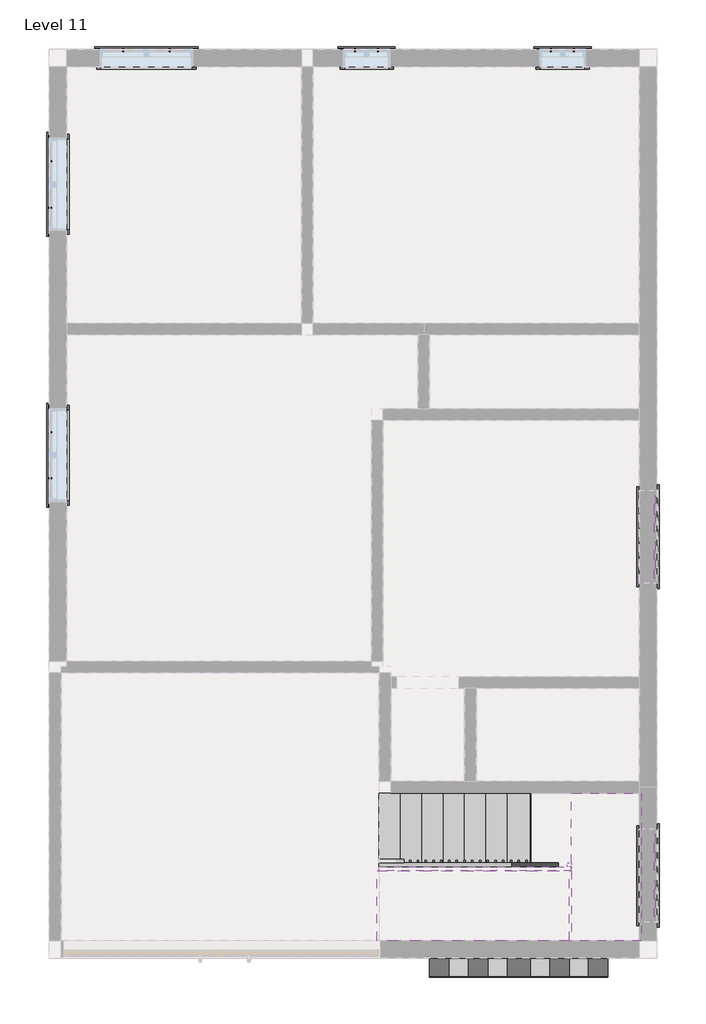
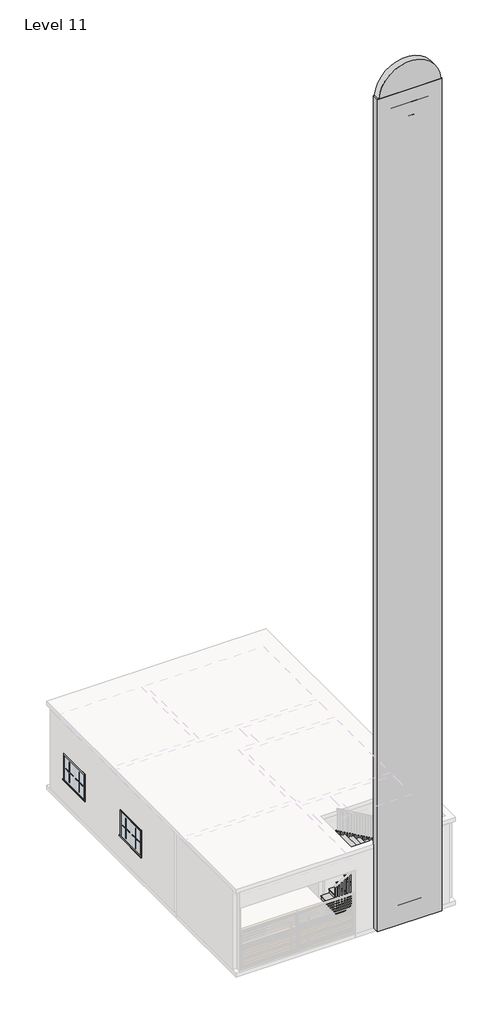
# One storey, part 3 of 3: 45 proxies, 6 members, 4 stair flights, 2 slabs.
"""IFC4 building model written with IfcOpenShell, lengths in millimetres."""

from ifc_helpers import new_model, si_unit, frame, origin, place, context, project, spatial, polyline, outline, extrude, transform, mapped, element, save
from components import generic_models_1_generic_models_1_ee720f7e, muntin_pattern_2x2_muntin_pattern_2x2_2357e71d, muntin_pattern_2x2_muntin_pattern_2x2_302d8f29, muntin_pattern_2x2_muntin_pattern_2x2_53152e2c, muntin_pattern_2x2_muntin_pattern_2x2_e8f3e573, trim_window_exterior_flat_with_sill_c4e67c73, trim_window_exterior_flat_with_sill_a665a915, trim_window_interior_flat_picture_frame_cf1733af, trim_window_interior_flat_picture_frame_d485c387, non_monolithic_landing_51f18b7d, stair_flight_922384ce, stair_flight_035a5224

model = new_model("IFC4")

# Units and contexts
model_context = context("Model", 3, world=origin())
ifc_project = project(units=[si_unit("LENGTHUNIT", "METRE", prefix="MILLI")], contexts=[model_context])

# Site, building, storey
site = spatial("IfcSite", under=ifc_project)
building = spatial("IfcBuilding", under=site)
storey = spatial("IfcBuildingStorey", under=building, Name="Level 11", Elevation=0.0)

# Proxies
placement = place(None, origin())
generic_models_1_generic_models_1_shape = generic_models_1_generic_models_1_ee720f7e(model_context)
element("IfcBuildingElementProxy", 1, Name="Generic Models 1 : Generic Models 1", ObjectType="Generic Models 1 : Generic Models 1", at=placement, inside=storey, context=model_context, shape_type="MappedRepresentation", body=[
    mapped(generic_models_1_generic_models_1_shape, transform((0.0, 0.0, 0.0), x_axis=(1.0, 0.0, 0.0), y_axis=(0.0, 1.0, 0.0), z_axis=(0.0, 0.0, 1.0))),
])
muntin_pattern_2x2_muntin_pattern_2x2_shape = muntin_pattern_2x2_muntin_pattern_2x2_2357e71d(model_context)
element("IfcBuildingElementProxy", 2, Name="Muntin Pattern_2x2 : Muntin Pattern_2x2", ObjectType="Muntin Pattern_2x2 : Muntin Pattern_2x2", at=placement, inside=storey, context=model_context, shape_type="MappedRepresentation", body=[
    mapped(muntin_pattern_2x2_muntin_pattern_2x2_shape, transform((-4942.3279463, 5897.3080275, 984.25), x_axis=(1.0, 0.0, 0.0), y_axis=(0.0, 1.0, 0.0), z_axis=(0.0, 0.0, 1.0))),
])
element("IfcBuildingElementProxy", 3, Name="Muntin Pattern_2x2 : Muntin Pattern_2x2", ObjectType="Muntin Pattern_2x2 : Muntin Pattern_2x2", at=placement, inside=storey, context=model_context, shape_type="MappedRepresentation", body=[
    mapped(muntin_pattern_2x2_muntin_pattern_2x2_shape, transform((-5899.5904463, 3838.3205275, 984.25), x_axis=(0.0, 1.0, 0.0), y_axis=(-1.0, 0.0, 0.0), z_axis=(0.0, 0.0, 1.0))),
])
element("IfcBuildingElementProxy", 4, Name="Muntin Pattern_2x2 : Muntin Pattern_2x2", ObjectType="Muntin Pattern_2x2 : Muntin Pattern_2x2", at=placement, inside=storey, context=model_context, shape_type="MappedRepresentation", body=[
    mapped(muntin_pattern_2x2_muntin_pattern_2x2_shape, transform((-5899.5904463, 293.4330275, 984.25), x_axis=(0.0, 1.0, 0.0), y_axis=(-1.0, 0.0, 0.0), z_axis=(0.0, 0.0, 1.0))),
])
element("IfcBuildingElementProxy", 5, Name="Muntin Pattern_2x2 : Muntin Pattern_2x2", ObjectType="Muntin Pattern_2x2 : Muntin Pattern_2x2", at=placement, inside=storey, context=model_context, shape_type="MappedRepresentation", body=[
    mapped(muntin_pattern_2x2_muntin_pattern_2x2_shape, transform((2031.5595537, -166.9419725, 1289.05), x_axis=(0.0, -1.0, 0.0), y_axis=(1.0, 0.0, 0.0), z_axis=(0.0, 0.0, 1.0))),
])
element("IfcBuildingElementProxy", 6, Name="Muntin Pattern_2x2 : Muntin Pattern_2x2", ObjectType="Muntin Pattern_2x2 : Muntin Pattern_2x2", at=placement, inside=storey, context=model_context, shape_type="MappedRepresentation", body=[
    mapped(muntin_pattern_2x2_muntin_pattern_2x2_shape, transform((2031.5595537, -4599.2419725, 1289.05), x_axis=(0.0, -1.0, 0.0), y_axis=(1.0, 0.0, 0.0), z_axis=(0.0, 0.0, 1.0))),
])
element("IfcBuildingElementProxy", 7, Name="Muntin Pattern_2x2 : Muntin Pattern_2x2", ObjectType="Muntin Pattern_2x2 : Muntin Pattern_2x2", at=placement, inside=storey, context=model_context, shape_type="MappedRepresentation", body=[
    mapped(muntin_pattern_2x2_muntin_pattern_2x2_shape, transform((-4942.3279463, 5897.3080275, 984.25), x_axis=(1.0, 0.0, 0.0), y_axis=(0.0, 1.0, 0.0), z_axis=(0.0, 0.0, 1.0))),
])
element("IfcBuildingElementProxy", 8, Name="Muntin Pattern_2x2 : Muntin Pattern_2x2", ObjectType="Muntin Pattern_2x2 : Muntin Pattern_2x2", at=placement, inside=storey, context=model_context, shape_type="MappedRepresentation", body=[
    mapped(muntin_pattern_2x2_muntin_pattern_2x2_shape, transform((2031.5595537, -4599.2419725, 1289.05), x_axis=(0.0, -1.0, 0.0), y_axis=(1.0, 0.0, 0.0), z_axis=(0.0, 0.0, 1.0))),
])
muntin_pattern_2x2_muntin_pattern_2x2_2_shape = muntin_pattern_2x2_muntin_pattern_2x2_302d8f29(model_context)
element("IfcBuildingElementProxy", 9, Name="Muntin Pattern_2x2 : Muntin Pattern_2x2", ObjectType="Muntin Pattern_2x2 : Muntin Pattern_2x2", at=placement, inside=storey, context=model_context, shape_type="MappedRepresentation", body=[
    mapped(muntin_pattern_2x2_muntin_pattern_2x2_2_shape, transform((-4335.9029463, 5897.3080275, 984.25), x_axis=(-1.0, 0.0, 0.0), y_axis=(0.0, -1.0, 0.0), z_axis=(0.0, 0.0, 1.0))),
])
element("IfcBuildingElementProxy", 10, Name="Muntin Pattern_2x2 : Muntin Pattern_2x2", ObjectType="Muntin Pattern_2x2 : Muntin Pattern_2x2", at=placement, inside=storey, context=model_context, shape_type="MappedRepresentation", body=[
    mapped(muntin_pattern_2x2_muntin_pattern_2x2_2_shape, transform((-5899.5904463, 4444.7455275, 984.25), x_axis=(0.0, -1.0, 0.0), y_axis=(1.0, 0.0, 0.0), z_axis=(0.0, 0.0, 1.0))),
])
element("IfcBuildingElementProxy", 11, Name="Muntin Pattern_2x2 : Muntin Pattern_2x2", ObjectType="Muntin Pattern_2x2 : Muntin Pattern_2x2", at=placement, inside=storey, context=model_context, shape_type="MappedRepresentation", body=[
    mapped(muntin_pattern_2x2_muntin_pattern_2x2_2_shape, transform((-5899.5904463, 899.8580275, 984.25), x_axis=(0.0, -1.0, 0.0), y_axis=(1.0, 0.0, 0.0), z_axis=(0.0, 0.0, 1.0))),
])
element("IfcBuildingElementProxy", 12, Name="Muntin Pattern_2x2 : Muntin Pattern_2x2", ObjectType="Muntin Pattern_2x2 : Muntin Pattern_2x2", at=placement, inside=storey, context=model_context, shape_type="MappedRepresentation", body=[
    mapped(muntin_pattern_2x2_muntin_pattern_2x2_2_shape, transform((2031.5595537, -773.3669725, 1289.05), x_axis=(0.0, 1.0, 0.0), y_axis=(-1.0, 0.0, 0.0), z_axis=(0.0, 0.0, 1.0))),
])
element("IfcBuildingElementProxy", 13, Name="Muntin Pattern_2x2 : Muntin Pattern_2x2", ObjectType="Muntin Pattern_2x2 : Muntin Pattern_2x2", at=placement, inside=storey, context=model_context, shape_type="MappedRepresentation", body=[
    mapped(muntin_pattern_2x2_muntin_pattern_2x2_2_shape, transform((2031.5595537, -5205.6669725, 1289.05), x_axis=(0.0, 1.0, 0.0), y_axis=(-1.0, 0.0, 0.0), z_axis=(0.0, 0.0, 1.0))),
])
element("IfcBuildingElementProxy", 14, Name="Muntin Pattern_2x2 : Muntin Pattern_2x2", ObjectType="Muntin Pattern_2x2 : Muntin Pattern_2x2", at=placement, inside=storey, context=model_context, shape_type="MappedRepresentation", body=[
    mapped(muntin_pattern_2x2_muntin_pattern_2x2_2_shape, transform((-4335.9029463, 5897.3080275, 984.25), x_axis=(-1.0, 0.0, 0.0), y_axis=(0.0, -1.0, 0.0), z_axis=(0.0, 0.0, 1.0))),
])
element("IfcBuildingElementProxy", 15, Name="Muntin Pattern_2x2 : Muntin Pattern_2x2", ObjectType="Muntin Pattern_2x2 : Muntin Pattern_2x2", at=placement, inside=storey, context=model_context, shape_type="MappedRepresentation", body=[
    mapped(muntin_pattern_2x2_muntin_pattern_2x2_2_shape, transform((2031.5595537, -5205.6669725, 1289.05), x_axis=(0.0, 1.0, 0.0), y_axis=(-1.0, 0.0, 0.0), z_axis=(0.0, 0.0, 1.0))),
])
muntin_pattern_2x2_muntin_pattern_2x2_3_shape = muntin_pattern_2x2_muntin_pattern_2x2_53152e2c(model_context)
element("IfcBuildingElementProxy", 16, Name="Muntin Pattern_2x2 : Muntin Pattern_2x2", ObjectType="Muntin Pattern_2x2 : Muntin Pattern_2x2", at=placement, inside=storey, context=model_context, shape_type="MappedRepresentation", body=[
    mapped(muntin_pattern_2x2_muntin_pattern_2x2_3_shape, transform((-1907.0279463, 5897.3080275, 984.25), x_axis=(1.0, 0.0, 0.0), y_axis=(0.0, 1.0, 0.0), z_axis=(0.0, 0.0, 1.0))),
])
element("IfcBuildingElementProxy", 17, Name="Muntin Pattern_2x2 : Muntin Pattern_2x2", ObjectType="Muntin Pattern_2x2 : Muntin Pattern_2x2", at=placement, inside=storey, context=model_context, shape_type="MappedRepresentation", body=[
    mapped(muntin_pattern_2x2_muntin_pattern_2x2_3_shape, transform((658.3720537, 5897.3080275, 984.25), x_axis=(1.0, 0.0, 0.0), y_axis=(0.0, 1.0, 0.0), z_axis=(0.0, 0.0, 1.0))),
])
element("IfcBuildingElementProxy", 18, Name="Muntin Pattern_2x2 : Muntin Pattern_2x2", ObjectType="Muntin Pattern_2x2 : Muntin Pattern_2x2", at=placement, inside=storey, context=model_context, shape_type="MappedRepresentation", body=[
    mapped(muntin_pattern_2x2_muntin_pattern_2x2_3_shape, transform((-1907.0279463, 5897.3080275, 984.25), x_axis=(1.0, 0.0, 0.0), y_axis=(0.0, 1.0, 0.0), z_axis=(0.0, 0.0, 1.0))),
])
element("IfcBuildingElementProxy", 19, Name="Muntin Pattern_2x2 : Muntin Pattern_2x2", ObjectType="Muntin Pattern_2x2 : Muntin Pattern_2x2", at=placement, inside=storey, context=model_context, shape_type="MappedRepresentation", body=[
    mapped(muntin_pattern_2x2_muntin_pattern_2x2_3_shape, transform((658.3720537, 5897.3080275, 984.25), x_axis=(1.0, 0.0, 0.0), y_axis=(0.0, 1.0, 0.0), z_axis=(0.0, 0.0, 1.0))),
])
muntin_pattern_2x2_muntin_pattern_2x2_4_shape = muntin_pattern_2x2_muntin_pattern_2x2_e8f3e573(model_context)
element("IfcBuildingElementProxy", 20, Name="Muntin Pattern_2x2 : Muntin Pattern_2x2", ObjectType="Muntin Pattern_2x2 : Muntin Pattern_2x2", at=placement, inside=storey, context=model_context, shape_type="MappedRepresentation", body=[
    mapped(muntin_pattern_2x2_muntin_pattern_2x2_4_shape, transform((-1605.4029463, 5897.3080275, 984.25), x_axis=(-1.0, 0.0, 0.0), y_axis=(0.0, -1.0, 0.0), z_axis=(0.0, 0.0, 1.0))),
])
element("IfcBuildingElementProxy", 21, Name="Muntin Pattern_2x2 : Muntin Pattern_2x2", ObjectType="Muntin Pattern_2x2 : Muntin Pattern_2x2", at=placement, inside=storey, context=model_context, shape_type="MappedRepresentation", body=[
    mapped(muntin_pattern_2x2_muntin_pattern_2x2_4_shape, transform((959.9970537, 5897.3080275, 984.25), x_axis=(-1.0, 0.0, 0.0), y_axis=(0.0, -1.0, 0.0), z_axis=(0.0, 0.0, 1.0))),
])
element("IfcBuildingElementProxy", 22, Name="Muntin Pattern_2x2 : Muntin Pattern_2x2", ObjectType="Muntin Pattern_2x2 : Muntin Pattern_2x2", at=placement, inside=storey, context=model_context, shape_type="MappedRepresentation", body=[
    mapped(muntin_pattern_2x2_muntin_pattern_2x2_4_shape, transform((-1605.4029463, 5897.3080275, 984.25), x_axis=(-1.0, 0.0, 0.0), y_axis=(0.0, -1.0, 0.0), z_axis=(0.0, 0.0, 1.0))),
])
element("IfcBuildingElementProxy", 23, Name="Muntin Pattern_2x2 : Muntin Pattern_2x2", ObjectType="Muntin Pattern_2x2 : Muntin Pattern_2x2", at=placement, inside=storey, context=model_context, shape_type="MappedRepresentation", body=[
    mapped(muntin_pattern_2x2_muntin_pattern_2x2_4_shape, transform((959.9970537, 5897.3080275, 984.25), x_axis=(-1.0, 0.0, 0.0), y_axis=(0.0, -1.0, 0.0), z_axis=(0.0, 0.0, 1.0))),
])
trim_window_exterior_flat_with_sill_shape = trim_window_exterior_flat_with_sill_c4e67c73(model_context)
element("IfcBuildingElementProxy", 24, Name="Trim-Window-Exterior-Flat : with Sill", ObjectType="Trim-Window-Exterior-Flat : with Sill", at=placement, inside=storey, context=model_context, shape_type="MappedRepresentation", body=[
    mapped(trim_window_exterior_flat_with_sill_shape, transform((-4639.1154463, 5906.8330275, 1828.8), x_axis=(-1.0, 0.0, 0.0), y_axis=(0.0, 0.0, 1.0), z_axis=(0.0, 1.0, 0.0))),
])
element("IfcBuildingElementProxy", 25, Name="Trim-Window-Exterior-Flat : with Sill", ObjectType="Trim-Window-Exterior-Flat : with Sill", at=placement, inside=storey, context=model_context, shape_type="MappedRepresentation", body=[
    mapped(trim_window_exterior_flat_with_sill_shape, transform((-5909.1154463, 4141.5330275, 1828.8), x_axis=(0.0, -1.0, 0.0), y_axis=(0.0, 0.0, 1.0), z_axis=(-1.0, 0.0, 0.0))),
])
element("IfcBuildingElementProxy", 26, Name="Trim-Window-Exterior-Flat : with Sill", ObjectType="Trim-Window-Exterior-Flat : with Sill", at=placement, inside=storey, context=model_context, shape_type="MappedRepresentation", body=[
    mapped(trim_window_exterior_flat_with_sill_shape, transform((-5909.1154463, 596.6455275, 1828.8), x_axis=(0.0, -1.0, 0.0), y_axis=(0.0, 0.0, 1.0), z_axis=(-1.0, 0.0, 0.0))),
])
element("IfcBuildingElementProxy", 27, Name="Trim-Window-Exterior-Flat : with Sill", ObjectType="Trim-Window-Exterior-Flat : with Sill", at=placement, inside=storey, context=model_context, shape_type="MappedRepresentation", body=[
    mapped(trim_window_exterior_flat_with_sill_shape, transform((2041.0845537, -470.1544725, 2133.6), x_axis=(0.0, 1.0, 0.0), y_axis=(0.0, 0.0, 1.0), z_axis=(1.0, 0.0, 0.0))),
])
element("IfcBuildingElementProxy", 28, Name="Trim-Window-Exterior-Flat : with Sill", ObjectType="Trim-Window-Exterior-Flat : with Sill", at=placement, inside=storey, context=model_context, shape_type="MappedRepresentation", body=[
    mapped(trim_window_exterior_flat_with_sill_shape, transform((2041.0845537, -4902.4544725, 2133.6), x_axis=(0.0, 1.0, 0.0), y_axis=(0.0, 0.0, 1.0), z_axis=(1.0, 0.0, 0.0))),
])
element("IfcBuildingElementProxy", 29, Name="Trim-Window-Exterior-Flat : with Sill", ObjectType="Trim-Window-Exterior-Flat : with Sill", at=placement, inside=storey, context=model_context, shape_type="MappedRepresentation", body=[
    mapped(trim_window_exterior_flat_with_sill_shape, transform((-4639.1154463, 5906.8330275, 1828.8), x_axis=(-1.0, 0.0, 0.0), y_axis=(0.0, 0.0, 1.0), z_axis=(0.0, 1.0, 0.0))),
])
element("IfcBuildingElementProxy", 30, Name="Trim-Window-Exterior-Flat : with Sill", ObjectType="Trim-Window-Exterior-Flat : with Sill", at=placement, inside=storey, context=model_context, shape_type="MappedRepresentation", body=[
    mapped(trim_window_exterior_flat_with_sill_shape, transform((2041.0845537, -4902.4544725, 2133.6), x_axis=(0.0, 1.0, 0.0), y_axis=(0.0, 0.0, 1.0), z_axis=(1.0, 0.0, 0.0))),
])
trim_window_exterior_flat_with_sill_2_shape = trim_window_exterior_flat_with_sill_a665a915(model_context)
element("IfcBuildingElementProxy", 31, Name="Trim-Window-Exterior-Flat : with Sill", ObjectType="Trim-Window-Exterior-Flat : with Sill", at=placement, inside=storey, context=model_context, shape_type="MappedRepresentation", body=[
    mapped(trim_window_exterior_flat_with_sill_2_shape, transform((-1756.2154463, 5906.8330275, 1828.8), x_axis=(-1.0, 0.0, 0.0), y_axis=(0.0, 0.0, 1.0), z_axis=(0.0, 1.0, 0.0))),
])
element("IfcBuildingElementProxy", 32, Name="Trim-Window-Exterior-Flat : with Sill", ObjectType="Trim-Window-Exterior-Flat : with Sill", at=placement, inside=storey, context=model_context, shape_type="MappedRepresentation", body=[
    mapped(trim_window_exterior_flat_with_sill_2_shape, transform((809.1845537, 5906.8330275, 1828.8), x_axis=(-1.0, 0.0, 0.0), y_axis=(0.0, 0.0, 1.0), z_axis=(0.0, 1.0, 0.0))),
])
element("IfcBuildingElementProxy", 33, Name="Trim-Window-Exterior-Flat : with Sill", ObjectType="Trim-Window-Exterior-Flat : with Sill", at=placement, inside=storey, context=model_context, shape_type="MappedRepresentation", body=[
    mapped(trim_window_exterior_flat_with_sill_2_shape, transform((-1756.2154463, 5906.8330275, 1828.8), x_axis=(-1.0, 0.0, 0.0), y_axis=(0.0, 0.0, 1.0), z_axis=(0.0, 1.0, 0.0))),
])
element("IfcBuildingElementProxy", 34, Name="Trim-Window-Exterior-Flat : with Sill", ObjectType="Trim-Window-Exterior-Flat : with Sill", at=placement, inside=storey, context=model_context, shape_type="MappedRepresentation", body=[
    mapped(trim_window_exterior_flat_with_sill_2_shape, transform((809.1845537, 5906.8330275, 1828.8), x_axis=(-1.0, 0.0, 0.0), y_axis=(0.0, 0.0, 1.0), z_axis=(0.0, 1.0, 0.0))),
])
trim_window_interior_flat_picture_frame_shape = trim_window_interior_flat_picture_frame_cf1733af(model_context)
element("IfcBuildingElementProxy", 35, Name="Trim-Window-Interior-Flat : Picture Frame", ObjectType="Trim-Window-Interior-Flat : Picture Frame", at=placement, inside=storey, context=model_context, shape_type="MappedRepresentation", body=[
    mapped(trim_window_interior_flat_picture_frame_shape, transform((-4639.1154463, 5678.2330275, 1828.8), x_axis=(1.0, 0.0, 0.0), y_axis=(0.0, 0.0, 1.0), z_axis=(0.0, -1.0, 0.0))),
])
element("IfcBuildingElementProxy", 36, Name="Trim-Window-Interior-Flat : Picture Frame", ObjectType="Trim-Window-Interior-Flat : Picture Frame", at=placement, inside=storey, context=model_context, shape_type="MappedRepresentation", body=[
    mapped(trim_window_interior_flat_picture_frame_shape, transform((-5680.5154463, 4141.5330275, 1828.8), x_axis=(0.0, 1.0, 0.0), y_axis=(0.0, 0.0, 1.0), z_axis=(1.0, 0.0, 0.0))),
])
element("IfcBuildingElementProxy", 37, Name="Trim-Window-Interior-Flat : Picture Frame", ObjectType="Trim-Window-Interior-Flat : Picture Frame", at=placement, inside=storey, context=model_context, shape_type="MappedRepresentation", body=[
    mapped(trim_window_interior_flat_picture_frame_shape, transform((-5680.5154463, 596.6455275, 1828.8), x_axis=(0.0, 1.0, 0.0), y_axis=(0.0, 0.0, 1.0), z_axis=(1.0, 0.0, 0.0))),
])
element("IfcBuildingElementProxy", 38, Name="Trim-Window-Interior-Flat : Picture Frame", ObjectType="Trim-Window-Interior-Flat : Picture Frame", at=placement, inside=storey, context=model_context, shape_type="MappedRepresentation", body=[
    mapped(trim_window_interior_flat_picture_frame_shape, transform((1812.4845537, -470.1544725, 2133.6), x_axis=(0.0, -1.0, 0.0), y_axis=(0.0, 0.0, 1.0), z_axis=(-1.0, 0.0, 0.0))),
])
element("IfcBuildingElementProxy", 39, Name="Trim-Window-Interior-Flat : Picture Frame", ObjectType="Trim-Window-Interior-Flat : Picture Frame", at=placement, inside=storey, context=model_context, shape_type="MappedRepresentation", body=[
    mapped(trim_window_interior_flat_picture_frame_shape, transform((1812.4845537, -4902.4544725, 2133.6), x_axis=(0.0, -1.0, 0.0), y_axis=(0.0, 0.0, 1.0), z_axis=(-1.0, 0.0, 0.0))),
])
element("IfcBuildingElementProxy", 40, Name="Trim-Window-Interior-Flat : Picture Frame", ObjectType="Trim-Window-Interior-Flat : Picture Frame", at=placement, inside=storey, context=model_context, shape_type="MappedRepresentation", body=[
    mapped(trim_window_interior_flat_picture_frame_shape, transform((-4639.1154463, 5678.2330275, 1828.8), x_axis=(1.0, 0.0, 0.0), y_axis=(0.0, 0.0, 1.0), z_axis=(0.0, -1.0, 0.0))),
])
element("IfcBuildingElementProxy", 41, Name="Trim-Window-Interior-Flat : Picture Frame", ObjectType="Trim-Window-Interior-Flat : Picture Frame", at=placement, inside=storey, context=model_context, shape_type="MappedRepresentation", body=[
    mapped(trim_window_interior_flat_picture_frame_shape, transform((1812.4845537, -4902.4544725, 2133.6), x_axis=(0.0, -1.0, 0.0), y_axis=(0.0, 0.0, 1.0), z_axis=(-1.0, 0.0, 0.0))),
])
trim_window_interior_flat_picture_frame_2_shape = trim_window_interior_flat_picture_frame_d485c387(model_context)
element("IfcBuildingElementProxy", 42, Name="Trim-Window-Interior-Flat : Picture Frame", ObjectType="Trim-Window-Interior-Flat : Picture Frame", at=placement, inside=storey, context=model_context, shape_type="MappedRepresentation", body=[
    mapped(trim_window_interior_flat_picture_frame_2_shape, transform((-1756.2154463, 5678.2330275, 1828.8), x_axis=(1.0, 0.0, 0.0), y_axis=(0.0, 0.0, 1.0), z_axis=(0.0, -1.0, 0.0))),
])
element("IfcBuildingElementProxy", 43, Name="Trim-Window-Interior-Flat : Picture Frame", ObjectType="Trim-Window-Interior-Flat : Picture Frame", at=placement, inside=storey, context=model_context, shape_type="MappedRepresentation", body=[
    mapped(trim_window_interior_flat_picture_frame_2_shape, transform((809.1845537, 5678.2330275, 1828.8), x_axis=(1.0, 0.0, 0.0), y_axis=(0.0, 0.0, 1.0), z_axis=(0.0, -1.0, 0.0))),
])
element("IfcBuildingElementProxy", 44, Name="Trim-Window-Interior-Flat : Picture Frame", ObjectType="Trim-Window-Interior-Flat : Picture Frame", at=placement, inside=storey, context=model_context, shape_type="MappedRepresentation", body=[
    mapped(trim_window_interior_flat_picture_frame_2_shape, transform((-1756.2154463, 5678.2330275, 1828.8), x_axis=(1.0, 0.0, 0.0), y_axis=(0.0, 0.0, 1.0), z_axis=(0.0, -1.0, 0.0))),
])
element("IfcBuildingElementProxy", 45, Name="Trim-Window-Interior-Flat : Picture Frame", ObjectType="Trim-Window-Interior-Flat : Picture Frame", at=placement, inside=storey, context=model_context, shape_type="MappedRepresentation", body=[
    mapped(trim_window_interior_flat_picture_frame_2_shape, transform((809.1845537, 5678.2330275, 1828.8), x_axis=(1.0, 0.0, 0.0), y_axis=(0.0, 0.0, 1.0), z_axis=(0.0, -1.0, 0.0))),
])

# Members
element("IfcMember", 46, ObjectType="Stringer - 2\" Width", at=placement, inside=storey, context=model_context, shape_type="SweptSolid", body=[
    extrude(outline(polyline([(209.0890626, -1591.1154463), (0.0, -1591.1154463), (0.0, -1342.8974141), (1268.924218, 872.6845537), (1620.1745172, 872.6845537), (209.0890626, -1591.1154463)])), frame((0.0, -4788.1544725, 0.0), z_axis=(0.0, 1.0, 0.0), x_axis=(0.0, 0.0, 1.0)), (0.0, 0.0, 1.0), 50.8),
])
element("IfcMember", 47, ObjectType="Stringer - 2\" Width", at=placement, inside=storey, context=model_context, shape_type="SweptSolid", body=[
    extrude(outline(polyline([(1458.0387634, 923.4845537), (1809.2890626, 923.4845537), (3249.4690626, -1591.1154463), (2898.2187634, -1591.1154463), (1458.0387634, 923.4845537)])), frame((0.0, -4838.9544725, 0.0), z_axis=(0.0, 1.0, 0.0), x_axis=(0.0, 0.0, 1.0)), (0.0, 0.0, 1.0), 50.8),
])
element("IfcMember", 48, ObjectType="Stringer - 2\" Width", at=placement, inside=storey, context=model_context, shape_type="SweptSolid", body=[
    extrude(outline(polyline([(872.6845537, -4737.3544725), (923.4845537, -4737.3544725), (923.4845537, -4788.1544725), (872.6845537, -4788.1544725), (872.6845537, -4737.3544725)])), frame((0.0, 0.0, 1371.6), z_axis=(0.0, 0.0, 1.0), x_axis=(1.0, 0.0, 0.0)), (0.0, 0.0, 1.0), 304.8),
])
element("IfcMember", 49, ObjectType="Stringer - 2\" Width", at=placement, inside=storey, context=model_context, shape_type="SweptSolid", body=[
    extrude(outline(polyline([(209.0890626, -1591.1154463), (0.0, -1591.1154463), (0.0, -1342.8974141), (1268.924218, 872.6845537), (1620.1745172, 872.6845537), (209.0890626, -1591.1154463)])), frame((0.0, -4788.1544725, 0.0), z_axis=(0.0, 1.0, 0.0), x_axis=(0.0, 0.0, 1.0)), (0.0, 0.0, 1.0), 50.8),
])
element("IfcMember", 50, ObjectType="Stringer - 2\" Width", at=placement, inside=storey, context=model_context, shape_type="SweptSolid", body=[
    extrude(outline(polyline([(1458.0387634, 923.4845537), (1809.2890626, 923.4845537), (3249.4690626, -1591.1154463), (2898.2187634, -1591.1154463), (1458.0387634, 923.4845537)])), frame((0.0, -4838.9544725, 0.0), z_axis=(0.0, 1.0, 0.0), x_axis=(0.0, 0.0, 1.0)), (0.0, 0.0, 1.0), 50.8),
])
element("IfcMember", 51, ObjectType="Stringer - 2\" Width", at=placement, inside=storey, context=model_context, shape_type="SweptSolid", body=[
    extrude(outline(polyline([(872.6845537, -4737.3544725), (923.4845537, -4737.3544725), (923.4845537, -4788.1544725), (872.6845537, -4788.1544725), (872.6845537, -4737.3544725)])), frame((0.0, 0.0, 1371.6), z_axis=(0.0, 0.0, 1.0), x_axis=(1.0, 0.0, 0.0)), (0.0, 0.0, 1.0), 304.8),
])

# Slabs
non_monolithic_landing_shape = non_monolithic_landing_51f18b7d(model_context)
element("IfcSlab", 52, ObjectType="Non-Monolithic Landing", at=placement, inside=storey, context=model_context, shape_type="MappedRepresentation", body=[
    mapped(non_monolithic_landing_shape, transform((0.0, 0.0, 0.0), x_axis=(1.0, 0.0, 0.0), y_axis=(0.0, 1.0, 0.0), z_axis=(0.0, 0.0, 1.0))),
])
element("IfcSlab", 53, ObjectType="Non-Monolithic Landing", at=placement, inside=storey, context=model_context, shape_type="MappedRepresentation", body=[
    mapped(non_monolithic_landing_shape, transform((0.0, 0.0, 0.0), x_axis=(1.0, 0.0, 0.0), y_axis=(0.0, 1.0, 0.0), z_axis=(0.0, 0.0, 1.0))),
])

# Stair flights
stair_flight_shape = stair_flight_922384ce(model_context)
element("IfcStairFlight", 54, ObjectType="2\" Tread 1\" Nosing 1/4\" Riser", at=placement, inside=storey, context=model_context, shape_type="MappedRepresentation", body=[
    mapped(stair_flight_shape, transform((0.0, 0.0, 0.0), x_axis=(1.0, 0.0, 0.0), y_axis=(0.0, 1.0, 0.0), z_axis=(0.0, 0.0, 1.0))),
])
stair_flight_2_shape = stair_flight_035a5224(model_context)
element("IfcStairFlight", 55, ObjectType="2\" Tread 1\" Nosing 1/4\" Riser", at=placement, inside=storey, context=model_context, shape_type="MappedRepresentation", body=[
    mapped(stair_flight_2_shape, transform((0.0, 0.0, 0.0), x_axis=(1.0, 0.0, 0.0), y_axis=(0.0, 1.0, 0.0), z_axis=(0.0, 0.0, 1.0))),
])
element("IfcStairFlight", 56, ObjectType="2\" Tread 1\" Nosing 1/4\" Riser", at=placement, inside=storey, context=model_context, shape_type="MappedRepresentation", body=[
    mapped(stair_flight_shape, transform((0.0, 0.0, 0.0), x_axis=(1.0, 0.0, 0.0), y_axis=(0.0, 1.0, 0.0), z_axis=(0.0, 0.0, 1.0))),
])
element("IfcStairFlight", 57, ObjectType="2\" Tread 1\" Nosing 1/4\" Riser", at=placement, inside=storey, context=model_context, shape_type="MappedRepresentation", body=[
    mapped(stair_flight_2_shape, transform((0.0, 0.0, 0.0), x_axis=(1.0, 0.0, 0.0), y_axis=(0.0, 1.0, 0.0), z_axis=(0.0, 0.0, 1.0))),
])

save(model, "model.ifc")

# Revit data of these elements
# Type "Muntin Pattern_2x2 : Muntin Pattern_2x2"
#   Width [instance default] = 4' - 0"
#   Thickness = 0' - 0 1/2"
#   Height [instance default] = 4' - 0"
#   Distance = 0' - 0 3/4"
#   Interior Material [instance default] = none
#   Exterior Material [instance default] = none
#   Default Elevation = 0
# Type "Trim-Window-Exterior-Flat : with Sill"
#   Trim Width = 0' - 2 1/4"
#   Trim Thickness_Picture Frame = 0' - 1 1/4"
#   Trim Thickness_with Sill = 0' - 0 3/4"
#   Sill Thickness = 0' - 1 1/4"
#   Opening Width [instance default] = 2' - 0"
#   Opening Height [instance default] = 3' - 0"
#   Default Elevation = 4' - 0"
#   Sill = yes
#   Picture Frame = no
#   Trim Material [instance default] = none
# Type "Trim-Window-Interior-Flat : Picture Frame"
#   Trim Thickness_Picture Frame = 0' - 1 1/4"
#   Trim Width = 0' - 2 1/4"
#   Trim Thickness_with Sill = 0' - 0 3/4"
#   Sill Thickness = 0' - 1 1/4"
#   Opening Width [instance default] = 2' - 0"
#   Opening Height [instance default] = 3' - 0"
#   Default Elevation = 4' - 0"
#   Sill = no
#   Picture Frame = yes
#   Trim Material [instance default] = none
# Element 1 (IfcBuildingElementProxy, "Generic Models 1 : Generic Models 1")
#   Phase Created = New Construction
#   Materials on its faces: "Brick, Common", "Gypsum Wall Board", "MARBLE"
# Elements 2, 3, 4, 5, 6, 7, 8, 9, 10, 11, 12, 13, 14, 15 (IfcBuildingElementProxy, "Muntin Pattern_2x2 : Muntin Pattern_2x2")
#   Width = 1' - 6 5/8"
#   Height = 2' - 6 1/2"
#   Interior Material = Wood - Stained
#   Exterior Material = Clad - White
#   Phase Created = New Construction
#   Materials on its faces: "Clad - White", "Wood - Stained"
# Elements 16, 17, 18, 19, 20, 21, 22, 23 (IfcBuildingElementProxy, "Muntin Pattern_2x2 : Muntin Pattern_2x2")
#   Width = 0' - 6 5/8"
#   Height = 2' - 6 1/2"
#   Interior Material = Wood - Stained
#   Exterior Material = Clad - White
#   Phase Created = New Construction
#   Materials on its faces: "Clad - White", "Wood - Stained"
# Elements 24, 25, 26, 27, 28, 29, 30 (IfcBuildingElementProxy, "Trim-Window-Exterior-Flat : with Sill")
#   Opening Width = 4' - 0"
#   Opening Height = 3' - 0"
#   Trim Material = Clad - White
#   Phase Created = New Construction
#   Materials on its faces: "Clad - White"
# Elements 31, 32, 33, 34 (IfcBuildingElementProxy, "Trim-Window-Exterior-Flat : with Sill")
#   Opening Width = 2' - 0"
#   Opening Height = 3' - 0"
#   Trim Material = Clad - White
#   Phase Created = New Construction
#   Materials on its faces: "Clad - White"
# Elements 35, 36, 37, 38, 39, 40, 41 (IfcBuildingElementProxy, "Trim-Window-Interior-Flat : Picture Frame")
#   Opening Width = 4' - 0"
#   Opening Height = 3' - 0"
#   Trim Material = Wood - Stained
#   Phase Created = New Construction
#   Materials on its faces: "Wood - Stained"
# Elements 42, 43, 44, 45 (IfcBuildingElementProxy, "Trim-Window-Interior-Flat : Picture Frame")
#   Opening Width = 2' - 0"
#   Opening Height = 3' - 0"
#   Trim Material = Wood - Stained
#   Phase Created = New Construction
#   Materials on its faces: "Wood - Stained"
# Elements 46, 47, 48, 49, 50, 51 (IfcMember, "Stringer - 2\" Width")
#   Phase Created = New Construction
# Elements 52, 53 (IfcSlab, "Non-Monolithic Landing")
#   Phase Created = New Construction
# Elements 54, 55, 56, 57 (IfcStairFlight, "2\" Tread 1\" Nosing 1/4\" Riser")
#   Phase Created = New Construction
# Materials
#   "Brick, Common": class "Masonry", colour RGB 170 98 104, transparency 0, Description = "Common brick", Cost = 0
#   "Gypsum Wall Board": class "Generic", colour RGB 127 127 127, transparency 0, Description = "Gypsum Wall Board", Cost = 0
#   "MARBLE": class "Generic", colour RGB 120 120 120, transparency 0, Cost = 0
#   "Clad - White": class "Wood", colour RGB 242 242 238, transparency 0, Cost = 0
#   "Wood - Stained": class "Wood", colour RGB 224 178 126, transparency 0, Cost = 0
